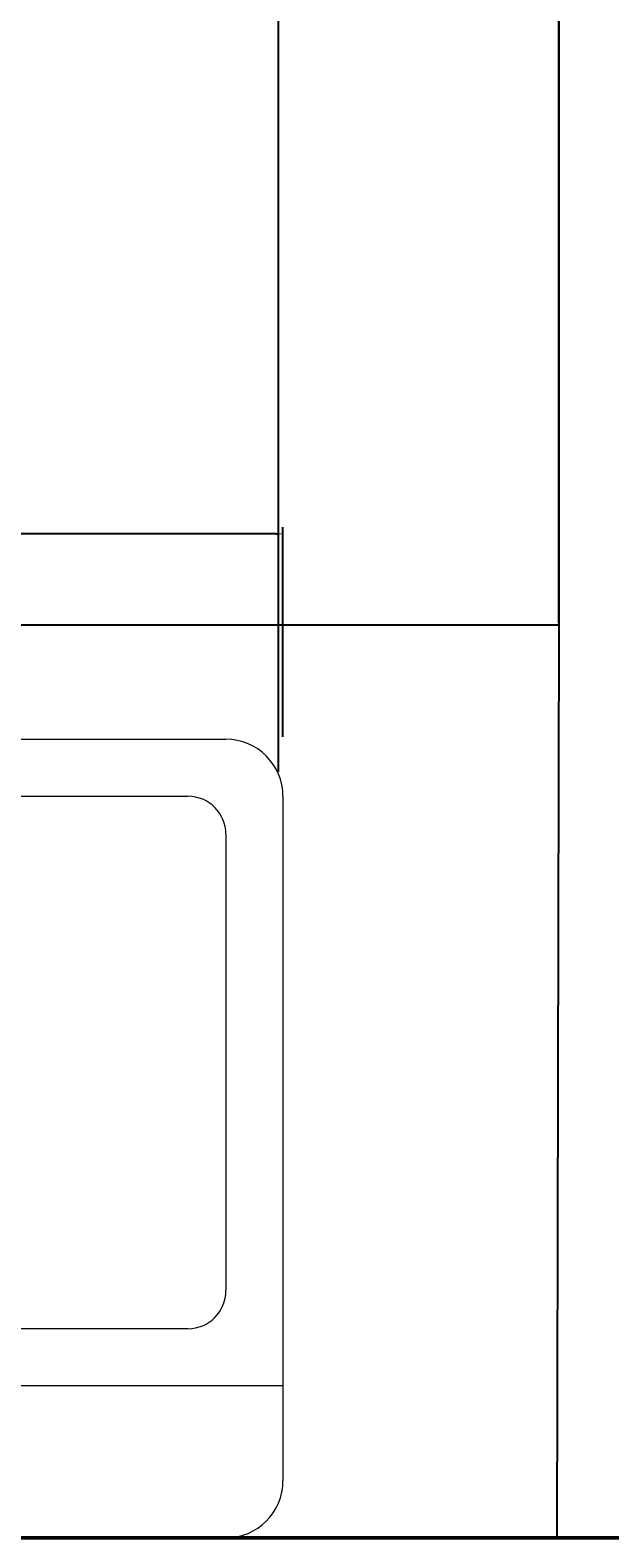
# Model space of a CAD drawing. Units: inches. Extents: x 2231 to 2461, y 2045 to 2455.
# Tile 21 of 95: x 2395 to 2410, y 2073 to 2112. Entities that reach past the tile are written whole.
import ezdxf

# ---------------------------------------------------------------- set-up
doc = ezdxf.new("R2010")
doc.units = ezdxf.units.IN
for name, color, linetype, lineweight in [('A-ANNO-DIMS', 2, 'Continuous', 18), ('A-FLOR-CASE', 8, 'Continuous', 25), ('A-FLOR-FIXT', 9, 'Continuous', 18), ('A-WALL', 7, 'Continuous', 50)]:
    doc.layers.add(name, color=color, linetype=linetype, lineweight=lineweight)
doc.styles.get("Standard").update_dxf_attribs({"font": 'arial.ttf'})
doc.dimstyles.get("Standard").update_dxf_attribs({"dimtxt": 0.18, "dimasz": 0.18, "dimexe": 0.18, "dimexo": 0.0625, "dimgap": 0.09, "dimtad": 0, "dimtih": 1, "dimtoh": 1, "dimdec": 4, "dimzin": 0, "dimdsep": 46, "dimtxsty": 'Standard', "dimcen": 0.09, "dimadec": 0, "dimazin": 0, "dimtfac": 1, "dimtdec": 4, "dimtofl": 0, "dimtmove": 0, "dimatfit": 3, "dimfxl": 1, "dimtolj": 1, "dimtzin": 0, "dimarcsym": 0})

# ---------------------------------------------------------------- blocks, each defined once
blk = doc.blocks.new('Sink-double - 36 in top')
for p, q in [((-18, -4), (18, -4)), ((-0.75, -18.5), (-0.75, -6.5)), ((0.75, -6.5), (0.75, -18.5))]:
    blk.add_line(p, q)
for points in [[(-16.5, 0), (16.5, 0)], [(-18, -19.5), (-18, -1.5)], [(18, -1.5), (18, -19.5)], [(-15.5, -5.5), (-1.75, -5.5)], [(1.75, -5.5), (15.5, -5.5)], [(-16.5, -18.5), (-16.5, -6.5)], [(16.5, -6.5), (16.5, -18.5)], [(-1.75, -19.5), (-15.5, -19.5)], [(15.5, -19.5), (1.75, -19.5)], [(16.5, -21), (-16.5, -21)]]:
    blk.add_lwpolyline(points)
for centre, radius in [((-8.5, -12.5), 1), ((8.5, -12.5), 1), ((-8.5, -12.5), 0.5), ((8.5, -12.5), 0.5)]:
    blk.add_circle(centre, radius)
for centre, radius, start, end in [((-16.5, -1.5), 1.5, 90, 180), ((16.5, -1.5), 1.5, 0, 90), ((-15.5, -6.5), 1, 90, 180), ((-1.75, -6.5), 1, 0, 90), ((1.75, -6.5), 1, 90, 180), ((15.5, -6.5), 1, 0, 90), ((-15.5, -18.5), 1, 180, 270), ((-1.75, -18.5), 1, 270, 0), ((1.75, -18.5), 1, 180, 270), ((15.5, -18.5), 1, 270, 0), ((-16.5, -19.5), 1.5, 180, 270), ((16.5, -19.5), 1.5, 270, 0)]:
    blk.add_arc(centre, radius, start, end)
blk = doc.blocks.new('*D29')
at = {"layer": 'A-ANNO-DIMS', "color": 0, "lineweight": -2, "transparency": 16777216}
for p, q in [((2365.54, 2093.895), (2365.54, 2099.413)), ((2401.54, 2093.895), (2401.54, 2099.413)), ((2365.72, 2099.233), (2382.993, 2099.233)), ((2401.36, 2099.233), (2384.087, 2099.233))]:
    blk.add_line(p, q, dxfattribs=at)
at = {"layer": 'A-ANNO-DIMS', "color": 0, "transparency": 16777216}
for points in [[(2365.72, 2099.263), (2365.72, 2099.203), (2365.54, 2099.233)], [(2401.36, 2099.263), (2401.36, 2099.203), (2401.54, 2099.233)]]:
    blk.add_solid(points, dxfattribs=at)
at = {"layer": 'Defpoints', "color": 0, "transparency": 16777216}
for p in [(2365.54, 2099.233), (2365.54, 2093.833), (2401.54, 2093.833)]:
    blk.add_point(p, dxfattribs=at)
at = {"layer": 'A-ANNO-DIMS', "color": 0, "transparency": 16777216, "insert": (2383.54, 2099.233), "char_height": 0.18, "attachment_point": 5}
blk.add_mtext('\\A1;SINK 36', dxfattribs=at)
blk = doc.blocks.new('*D66')
at = {"layer": 'A-ANNO-DIMS', "color": 0, "lineweight": -2, "transparency": 16777216}
for p, q in [((2348.189, 2096.895), (2348.189, 2454.645)), ((2408.794, 2096.895), (2408.794, 2454.645)), ((2348.369, 2454.465), (2378.167, 2454.465)), ((2408.614, 2454.465), (2378.815, 2454.465))]:
    blk.add_line(p, q, dxfattribs=at)
at = {"layer": 'A-ANNO-DIMS', "color": 0, "transparency": 16777216}
for points in [[(2348.369, 2454.495), (2348.369, 2454.435), (2348.189, 2454.465)], [(2408.614, 2454.495), (2408.614, 2454.435), (2408.794, 2454.465)]]:
    blk.add_solid(points, dxfattribs=at)
at = {"layer": 'Defpoints', "color": 0, "transparency": 16777216}
for p in [(2408.794, 2454.465), (2348.189, 2096.833), (2408.794, 2096.833)]:
    blk.add_point(p, dxfattribs=at)
at = {"layer": 'A-ANNO-DIMS', "color": 0, "transparency": 16777216, "insert": (2378.491, 2454.465), "char_height": 0.18, "attachment_point": 5}
blk.add_mtext('\\A1;60.6', dxfattribs=at)
blk = doc.blocks.new('*D71')
at = {"layer": 'A-ANNO-DIMS', "color": 0, "lineweight": -2, "transparency": 16777216}
for p, q in [((2401.422, 2092.979), (2401.422, 2454.645)), ((2408.794, 2096.895), (2408.794, 2454.645)), ((2401.602, 2454.465), (2404.732, 2454.465)), ((2408.614, 2454.465), (2405.483, 2454.465))]:
    blk.add_line(p, q, dxfattribs=at)
at = {"layer": 'A-ANNO-DIMS', "color": 0, "transparency": 16777216}
for points in [[(2401.602, 2454.495), (2401.602, 2454.435), (2401.422, 2454.465)], [(2408.614, 2454.495), (2408.614, 2454.435), (2408.794, 2454.465)]]:
    blk.add_solid(points, dxfattribs=at)
at = {"layer": 'Defpoints', "color": 0, "transparency": 16777216}
for p in [(2408.794, 2454.465), (2408.794, 2096.833), (2401.422, 2092.917)]:
    blk.add_point(p, dxfattribs=at)
at = {"layer": 'A-ANNO-DIMS', "color": 0, "transparency": 16777216, "insert": (2405.108, 2454.465), "char_height": 0.18, "attachment_point": 5}
blk.add_mtext('\\A1;7.371', dxfattribs=at)

msp = doc.modelspace()

# ---------------------------------------------------------------- linework, layer by layer
at = {"layer": 'A-FLOR-CASE'}
for p, q in [((2408.7935, 2182.8328), (2408.7935, 2096.8328)), ((2408.7935, 2096.8328), (2348.1888, 2096.8328)), ((2408.7935, 2096.8328), (2408.7447, 2072.8328))]:
    msp.add_line(p, q, dxfattribs=at)
at = {"layer": 'A-WALL'}
msp.add_line((2432.7935, 2072.8328), (2330.7942, 2072.8328), dxfattribs=at)

# ---------------------------------------------------------------- block references
at = {"layer": 'A-FLOR-FIXT', "rotation": 180}
msp.add_blockref('Sink-double - 36 in top', (2383.54, 2072.8328), dxfattribs=at)

# ---------------------------------------------------------------- dimensions: what is measured, and where the dimension line sits
at = {"layer": 'A-ANNO-DIMS'}
for p1, override, picture, middle in [((2348.1888, 2096.8328), {"dimdec": 1, "dimlfac": 1, "dimrnd": 0, "dimzin": 0, "dimdsep": 46, "dimlunit": 2}, '*D66', (2378.4912, 2454.4653)), ((2401.4221, 2092.9167), {"dimdec": 3, "dimlfac": 1, "dimrnd": 0, "dimzin": 0, "dimdsep": 46, "dimlunit": 2}, '*D71', (2405.1078, 2454.4653))]:
    dim = msp.add_linear_dim(base=(2408.7935, 2454.4653), p1=p1, p2=(2408.7935, 2096.8328), dimstyle='Standard', override=override, dxfattribs=at)
    dim.commit()
    dim.dimension.update_dxf_attribs({"geometry": picture, "text_midpoint": middle})
dim = msp.add_linear_dim(base=(2365.54, 2099.2328), p1=(2401.54, 2093.8328), p2=(2365.54, 2093.8328), angle=180, text='SINK <>', dimstyle='Standard', override={"dimdec": 0, "dimlfac": 1, "dimrnd": 0, "dimzin": 0, "dimdsep": 46, "dimlunit": 2}, dxfattribs=at)
dim.commit()
dim.dimension.update_dxf_attribs({"geometry": '*D29', "text_midpoint": (2383.54, 2099.2328)})

doc.saveas('drawing.dxf')
